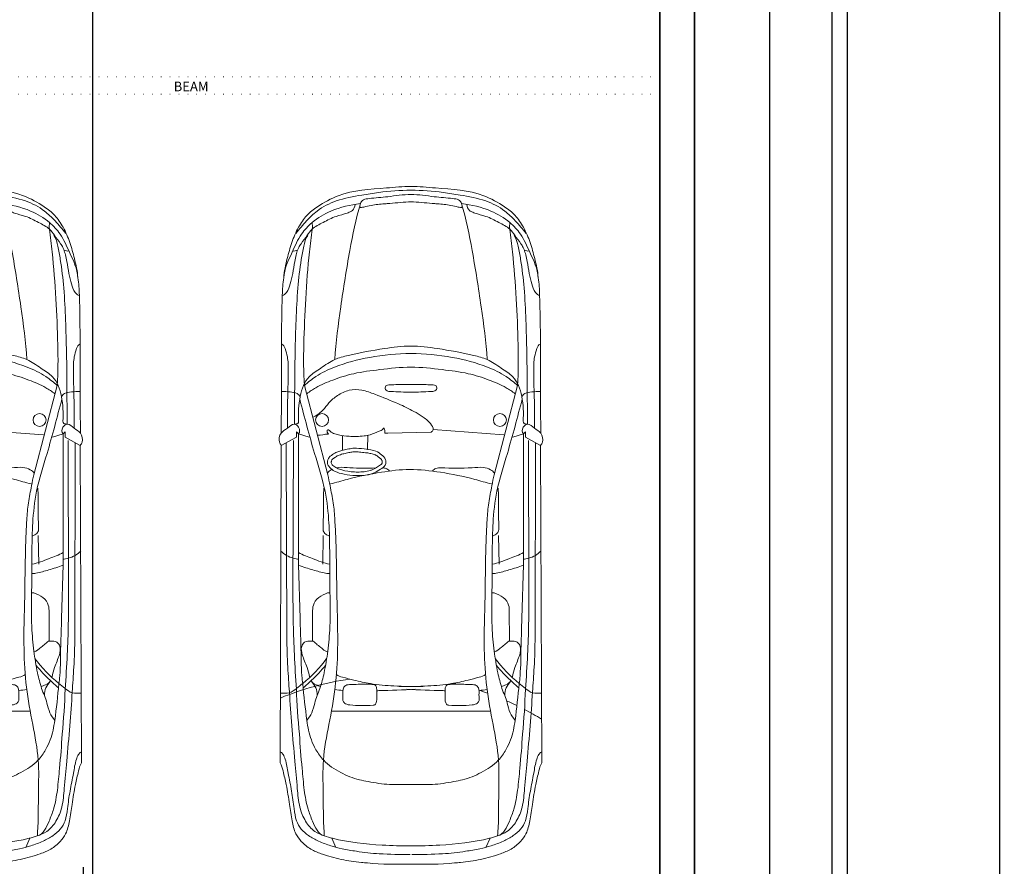
# Model space of a CAD drawing. Units: inches. Extents: x 1239 to 2276906, y 2273 to 321338.
# Tile 13 of 23: x 1754 to 2011, y 2429 to 2650. Entities that reach past the tile are written whole.
import ezdxf

# ---------------------------------------------------------------- set-up
doc = ezdxf.new("R2010")
doc.units = ezdxf.units.IN
doc.linetypes.add('DOT', pattern=[6.35, 0, -6.35])
for name, color, linetype, lineweight in [('A-ANNO-DIMS', 2, 'Continuous', 18), ('A-ANNO-TEXT', 7, 'Continuous', 18), ('BEAM LINE', 4, 'DOT', 18), ('C-PRKG', 8, 'Continuous', 13), ('C-PROP', 7, 'Continuous', 25), ('wall', 7, 'Continuous', 35)]:
    doc.layers.add(name, color=color, linetype=linetype, lineweight=lineweight)
doc.styles.get("Standard").update_dxf_attribs({"font": 'arial.ttf'})
doc.dimstyles.new('ISO-25', dxfattribs={"dimtxt": 4.5, "dimasz": 4, "dimexe": 1.25, "dimexo": 0.625, "dimtad": 1, "dimdec": 1, "dimlunit": 3, "dimtxsty": 'Standard', "dimcen": 2.5, "dimadec": 0, "dimazin": 0, "dimtfac": 1, "dimtdec": 1, "dimtmove": 0, "dimatfit": 3, "dimfxl": 1, "dimarcsym": 0})

# ---------------------------------------------------------------- blocks, each defined once
blk = doc.blocks.new('A$C242571DA')
for p, q in [((1659.9, 1632), (1714.3, 1732.5)), ((1699.9, 1699.4), (2984.7, 1695.8)), ((1714.3, 1732.5), (3817.1, 1739.9)), ((1638.3, 1618.5), (1625.1, 1632)), ((1625.1, 1632), (1659.9, 1632)), ((1681.8, 1651.6), (2695.2, 1655.3)), ((1317.4, 1579.7), (1909.8, 1424.9)), ((1638.3, 1618.5), (2503.3, 1618.5)), ((1659.9, 1548.1), (1638.3, 1618.5)), ((2503.3, 1618.5), (2861.6, 1607.5)), ((3007.2, 1526.5), (2808.1, 1525.2)), ((1644, 1489.1), (1610.4, 1020.2)), ((2311.9, 1454.3), (2500.6, 1456.9)), ((3474.6, 1401.1), (3474.6, 843)), ((4315.2, 1398), (4377.3, 1370.5)), ((1626.1, 1006.5), (1632.8, 719.7)), ((3474.6, 345.6), (3474.6, 903.8)), ((1740.2, 584.9), (1649.3, 586.9)), ((1746.1, 420.6), (1649.3, 420.6)), ((4315.2, 348.7), (4377.3, 376.3)), ((1317.4, 167), (1909.8, 321.9)), ((2311.9, 292.5), (2500.6, 289.8)), ((1659.9, 198.7), (1638.3, 128.2)), ((3007.2, 220.3), (2808.1, 221.6)), ((2503.3, 128.2), (2861.6, 139.2)), ((1638.3, 128.2), (1625.1, 114.7)), ((1625.1, 114.7), (1659.9, 114.7)), ((1638.3, 128.2), (2503.3, 128.2)), ((1659.9, 114.7), (1714.3, 14.2)), ((1681.8, 95.1), (2695.2, 91.4)), ((1699.9, 47.3), (2984.7, 51)), ((1714.3, 14.2), (3817.1, 6.9))]:
    blk.add_line(p, q)
for centre in [(1546.4, 1462.5), (1546.4, 284.2)]:
    blk.add_ellipse(centre, major_axis=(0, 42.9), ratio=0.983266, start_param=4.712389, end_param=10.995574)
for points, knots in [([(0, 873.4), (0, 927.8), (15.6, 1088.6), (25.5, 1309.8), (120.7, 1476.4), (189.2, 1569), (273.5, 1623.1), (369.9, 1666.3), (483, 1694.7), (561.3, 1714.9), (604.6, 1715.7)], [0, 0, 0, 0, 0.16039, 0.479033, 0.632967, 0.722015, 0.817474, 0.927562, 1.03733, 1.167094, 1.167094, 1.167094, 1.167094]), ([(604.6, 1715.7), (545.5, 1714.5), (448.5, 1664.6), (320.8, 1610.6), (225.4, 1521.2), (147.3, 1390.5), (121.7, 1275.2), (113.6, 1208.7)], [0, 0, 0, 0, 0.1772572, 0.3124951, 0.4151678, 0.5597243, 0.7575412, 0.7575412, 0.7575412, 0.7575412]), ([(722.7, 1726.6), (720.8, 1714.9), (694.5, 1689.9), (643, 1671.8), (573.6, 1655.4), (508.5, 1647), (455.2, 1634.7), (428.7, 1627.3), (416.9, 1624.1)], [0, 0, 0, 0, 0.034703, 0.0959761, 0.1659336, 0.2471559, 0.2929944, 0.3295918, 0.3295918, 0.3295918, 0.3295918]), ([(604.6, 1715.7), (642.1, 1723.4), (788.5, 1729.2), (1039.3, 1732.2), (1344.5, 1729.9), (1542, 1733.1), (1633.8, 1733.7)], [0, 0, 0, 0, 0.114897, 0.437061, 0.754269, 1.029686, 1.029686, 1.029686, 1.029686]), ([(1043.6, 1729.2), (1048.6, 1717.9), (1080.9, 1704.2), (1138.6, 1687.6), (1237.7, 1685.6), (1394.7, 1691.3), (1521.7, 1692.4), (1601.5, 1692.7)], [0, 0, 0, 0, 0.0364992, 0.0923739, 0.1867837, 0.3273982, 0.5667068, 0.5667068, 0.5667068, 0.5667068]), ([(1356.8, 1732.2), (1357.1, 1712.8), (1360, 1678.8), (1363.9, 1630.5), (1383.3, 1613.5), (1391, 1607.2)], [0, 0, 0, 0, 1.462159, 2.651105, 3.386321, 3.386321, 3.386321, 3.386321]), ([(1714.3, 1732.5), (1707.7, 1737.6), (1683.3, 1753), (1628.7, 1741.2), (1605.6, 1691.5), (1561.7, 1652.4), (1594.1, 1610.3), (1627.9, 1608.3), (1638.3, 1618.5)], [0, 0, 0, 0, 0.024864, 0.0846267, 0.1362471, 0.1900683, 0.2245199, 0.2681841, 0.2681841, 0.2681841, 0.2681841]), ([(2414.7, 1735), (2424.9, 1723.3), (2447.2, 1698.8), (2461.2, 1657.6), (2468.1, 1629), (2468, 1616.1)], [1.808086, 1.808086, 1.808086, 1.808086, 2.918874, 4.131288, 5.10151, 5.10151, 5.10151, 5.10151]), ([(3356.5, 1739.4), (3354.9, 1719.2), (3360.8, 1678.2), (3324, 1631.5), (3255.4, 1544.3), (3187.1, 1476.2), (3125.2, 1432.2)], [0, 0, 0, 0, 0.0597371, 0.1139981, 0.1672498, 0.3938869, 0.3938869, 0.3938869, 0.3938869]), ([(3745.3, 1736.8), (3748.5, 1730.1), (3764.2, 1717.1), (3811.5, 1698.6), (3894.7, 1686.7), (4002.9, 1663.2), (4107.9, 1648.7), (4195.8, 1638.3), (4258.6, 1603.2), (4302.1, 1549.7), (4339.9, 1483.8), (4365.2, 1407.6), (4389.6, 1324.4), (4397.9, 1266.9), (4401.8, 1235.2)], [0, 0, 0, 0, 0.0219205, 0.0572122, 0.1522539, 0.2718866, 0.3894011, 0.4710097, 0.5346344, 0.5986698, 0.6733118, 0.758696, 0.8351341, 0.9293726, 0.9293726, 0.9293726, 0.9293726]), ([(3817.1, 1739.9), (3833.2, 1729.7), (3882.9, 1718.2), (3973.3, 1695.2), (4085.1, 1680.5), (4193.8, 1662.8), (4280.6, 1644.3), (4343.9, 1598.1), (4390, 1540.3), (4427.4, 1448.7), (4457.8, 1336.6), (4475.7, 1233.4), (4478.4, 1175.1), (4479.3, 1161.6)], [0, 0, 0, 0, 0.056668, 0.14946, 0.28161, 0.392935, 0.481686, 0.542967, 0.622845, 0.69797, 0.833643, 0.965665, 1.00577, 1.00577, 1.00577, 1.00577]), ([(310.7, 1637.3), (282.5, 1613.7), (230.1, 1569.9), (148.7, 1486.2), (84.8, 1361.3), (60, 1219), (32.6, 1054.3), (25.1, 944.9), (25.1, 873.4)], [0, 0, 0, 0, 0.1095129, 0.2035347, 0.3452507, 0.5161382, 0.6275464, 0.8383798, 0.8383798, 0.8383798, 0.8383798]), ([(426.8, 1656.7), (428.5, 1646.6), (426.9, 1625), (399.8, 1616.6), (368.1, 1593.9), (328, 1564.6), (271.6, 1523.9), (237, 1451.9), (196.2, 1376.7), (183.8, 1314.9), (170, 1279.6), (157.2, 1254.2), (133.3, 1244.4), (118.6, 1242.9)], [0, 0, 0, 0, 0.0304541, 0.0502818, 0.0786089, 0.1479133, 0.1986294, 0.2831705, 0.3780326, 0.4523267, 0.4667809, 0.4902599, 0.5347198, 0.5347198, 0.5347198, 0.5347198]), ([(323.7, 1557.5), (344.8, 1571.9), (400.4, 1585.1), (516, 1606.8), (680.3, 1625.8), (885.4, 1635.7), (1116.8, 1642.2), (1346.1, 1644.2), (1504.7, 1644.7), (1574, 1645.7)], [0, 0, 0, 0, 0.076148, 0.165903, 0.355672, 0.569871, 0.782325, 1.050047, 1.257936, 1.257936, 1.257936, 1.257936]), ([(1574, 1645.7), (1572.9, 1638), (1574.1, 1622), (1559.9, 1618.7), (1555.2, 1617.8)], [0, 0, 0, 0, 0.02274132, 0.03717479, 0.03717479, 0.03717479, 0.03717479]), ([(2695.2, 1655.3), (2829.9, 1655.3), (3041.2, 1651.4), (3351.3, 1630.7), (3527.5, 1623.2), (3626.6, 1612)], [0, 0, 0, 0, 0.4042759, 0.6333827, 0.9326252, 0.9326252, 0.9326252, 0.9326252]), ([(2984.7, 1695.8), (3051, 1695.6), (3172.1, 1691.3), (3367.4, 1677.6), (3575.2, 1664.3), (3788.2, 1643.6), (3968, 1628.1), (4103.8, 1616.8), (4203.6, 1578.1), (4271.8, 1519.5), (4300.6, 1452.1), (4341.7, 1305.3), (4361.8, 1111.2), (4367.5, 936.8), (4367.5, 873.4)], [0, 0, 0, 0, 0.198873, 0.363323, 0.587433, 0.823543, 1.004622, 1.129816, 1.230113, 1.320655, 1.388577, 1.443334, 1.771447, 1.958652, 1.958652, 1.958652, 1.958652]), ([(1317.4, 1579.7), (1227.8, 1586.1), (1036, 1584.8), (741.2, 1572.5), (486.1, 1553.3), (333.3, 1534.3), (283.3, 1528.5)], [0, 0, 0, 0, 0.269375, 0.574535, 0.885339, 1.036319, 1.036319, 1.036319, 1.036319]), ([(1555.2, 1617.8), (1527.7, 1617.8), (1472.5, 1620.4), (1392.7, 1608.8), (1318.5, 1591), (1249.4, 1545.5), (1201.4, 1466.7), (1142.8, 1385.7), (1104.8, 1240.4), (1076, 1072.3), (1056.4, 932.4), (1056.4, 873.4)], [0, 0, 0, 0, 0.082256, 0.165174, 0.241383, 0.30939, 0.405348, 0.511507, 0.603349, 0.843635, 1.017671, 1.017671, 1.017671, 1.017671]), ([(1317.4, 1579.7), (1296.6, 1555.5), (1247.9, 1494.4), (1177.6, 1350.5), (1124.2, 1137.4), (1105.5, 964.9), (1105.5, 873.4)], [0, 0, 0, 0, 0.0947759, 0.2311242, 0.4700259, 0.7400315, 0.7400315, 0.7400315, 0.7400315]), ([(3535.9, 1563.1), (3520.1, 1550.9), (3484.4, 1526.1), (3408.2, 1510.9), (3323.4, 1473.1), (3207.9, 1445), (3072.6, 1422.2), (2866.9, 1404.6), (2626.4, 1412.9), (2396.7, 1410.8), (2200.9, 1416.9), (2001.3, 1438.2), (1732.1, 1525.9), (1527.9, 1578.9), (1407.5, 1610.7)], [0, 0, 0, 0, 0.05975, 0.126928, 0.230034, 0.336675, 0.482225, 0.641324, 0.954906, 1.203173, 1.330375, 1.542773, 1.802261, 2.175545, 2.175545, 2.175545, 2.175545]), ([(2424, 1618.7), (2441.5, 1589.9), (2464.2, 1518.9), (2495.4, 1450.9), (2501.6, 1411.3)], [0, 0, 0, 0, 0.1000351, 0.2184418, 0.2184418, 0.2184418, 0.2184418]), ([(2507.7, 1618.4), (2521, 1587.7), (2536.6, 1527.1), (2559.6, 1458.5), (2563.3, 1420.6), (2563.8, 1411.4)], [0, 0, 0, 0, 2.528586, 4.711885, 5.408215, 5.408215, 5.408215, 5.408215]), ([(2861.6, 1607.5), (2921.1, 1607.3), (3047.2, 1600.8), (3191.4, 1602), (3356.6, 1584.1), (3498.3, 1570.6), (3623.2, 1549.4), (3664.1, 1533.3)], [0, 0, 0, 0, 0.1783018, 0.3787173, 0.431954, 0.6762374, 0.8077184, 0.8077184, 0.8077184, 0.8077184]), ([(3248.1, 1545.2), (3226.9, 1550.4), (3176.1, 1562.1), (3113.7, 1592.9), (3052.6, 1605.3), (3010.4, 1578.8), (3010.3, 1545.3), (3010.3, 1515.9), (3033.7, 1500.1), (3052.6, 1465.2), (3078.9, 1443.5), (3084, 1424.4)], [0, 0, 0, 0, 0.0655106, 0.1550445, 0.2094604, 0.2438604, 0.287164, 0.3001388, 0.3275984, 0.3616951, 0.4200969, 0.4200969, 0.4200969, 0.4200969]), ([(3319, 1587.1), (3303.3, 1568.1), (3256.9, 1516.7), (3206.7, 1467.3), (3171.4, 1439.5)], [0, 0, 0, 0, 1.868162, 5.271297, 5.271297, 5.271297, 5.271297]), ([(3626.6, 1612), (3702.5, 1609.1), (3826.2, 1596.8), (3991.4, 1583.2), (4111.7, 1562.4), (4212.2, 1522.7), (4290.4, 1488), (4300.7, 1447.5)], [0, 0, 0, 0, 0.2277977, 0.3719478, 0.4996814, 0.5863441, 0.709615, 0.709615, 0.709615, 0.709615]), ([(1372.8, 1563.1), (1357.2, 1545), (1321.6, 1490.1), (1277, 1385.7), (1232.8, 1244.2), (1211.1, 1069.4), (1196.8, 942.4), (1196.8, 873.4)], [0, 0, 0, 0, 0.0708922, 0.1925846, 0.3348457, 0.5072814, 0.7109928, 0.7109928, 0.7109928, 0.7109928]), ([(2808.1, 1525.2), (2791.9, 1525.1), (2751.9, 1519.7), (2710.6, 1472.6), (2690, 1431.1), (2690.5, 1409.6)], [0, 0, 0, 0, 0.0486628, 0.1144515, 0.1777721, 0.1777721, 0.1777721, 0.1777721]), ([(3275.5, 1532.8), (3287.5, 1528.3), (3299.8, 1504.9), (3308.4, 1482.5), (3311.7, 1472.6)], [0, 0, 0, 0, 0.983949, 1.771691, 1.771691, 1.771691, 1.771691]), ([(3372.2, 1495.3), (3354.4, 1496.8), (3316, 1494.7), (3291.6, 1525.8), (3275.5, 1532.8)], [0, 0, 0, 0, 0.0535488, 0.1060573, 0.1060573, 0.1060573, 0.1060573]), ([(3664.1, 1533.3), (3687, 1526), (3734.8, 1502.3), (3816.7, 1444.8), (3884.1, 1342.9), (3925.1, 1239.9), (3937.3, 1177), (3940.4, 1157.6)], [0, 0, 0, 0, 0.0720749, 0.1581284, 0.2958089, 0.4262456, 0.4842292, 0.4842292, 0.4842292, 0.4842292]), ([(1909.8, 1424.9), (1933.5, 1418.7), (1995.6, 1407.6), (2094.4, 1385.8), (2211.8, 1377.1), (2419, 1366.9), (2704.7, 1366.5), (3032.7, 1354.2), (3316.2, 1371), (3558.7, 1415.9), (3789.1, 1461.7), (4028.9, 1452.9), (4196.2, 1455.2), (4292.7, 1447.9), (4300.7, 1447.5)], [0, 0, 0, 0, 0.073325, 0.188896, 0.303039, 0.425821, 0.811242, 1.159737, 1.41058, 1.660623, 1.899627, 2.11145, 2.377727, 2.401703, 2.401703, 2.401703, 2.401703]), ([(1997.2, 1450.5), (2039.7, 1454.5), (2126.7, 1451.9), (2219.8, 1454.5), (2287.1, 1456.9), (2305.7, 1434.4), (2313.2, 1419.9), (2315.8, 1413.5)], [0, 0, 0, 0, 3.267856, 6.568708, 7.399663, 8.099385, 8.621705, 8.621705, 8.621705, 8.621705]), ([(113.6, 1208.7), (215.2, 1238.6), (443.2, 1284.9), (788, 1338.7), (1029.5, 1370.7), (1146.4, 1378.6)], [0, 0, 0, 0, 0.317374, 0.69576, 1.04714, 1.04714, 1.04714, 1.04714]), ([(1898.5, 1426.2), (1889, 1420.6), (1871, 1397.2), (1856.4, 1345.2), (1867.7, 1233.5), (1864.3, 1132.3), (1863, 1038.5), (1876.9, 1022.3), (1884.5, 1015.7)], [0, 0, 0, 0, 0.842998, 2.122875, 3.997599, 9.174838, 10.012722, 10.751336, 10.751336, 10.751336, 10.751336]), ([(1969.6, 1407.3), (1960.5, 1369.8), (1927, 1259.1), (1890.9, 1078.4), (1874.3, 933), (1874.3, 864.4)], [0, 0, 0, 0, 0.1139079, 0.3411539, 0.543502, 0.543502, 0.543502, 0.543502]), ([(3231.5, 1368.3), (3240.8, 1356.2), (3253.1, 1315.7), (3271.9, 1240.7), (3297.9, 1127.9), (3310.5, 974.6), (3311.2, 858.3), (3311.6, 794.4)], [0, 0, 0, 0, 0.0451009, 0.1211996, 0.2308505, 0.385263, 0.5739042, 0.5739042, 0.5739042, 0.5739042]), ([(3294.8, 1174.5), (3294.8, 1207.4), (3299.6, 1249.5), (3298.3, 1303.9), (3326.3, 1329), (3363.9, 1320.7), (3399.3, 1329.3), (3422.1, 1315.7), (3430.7, 1297.9), (3438.7, 1234.2), (3439.6, 1174.4), (3434.7, 1112.2), (3418.9, 1102), (3395.9, 1098.6), (3362.6, 1100.9), (3331.1, 1096.6), (3298.8, 1107.6), (3297.3, 1140.3), (3294.8, 1160.9), (3294.8, 1174.5)], [0, 0, 0, 0, 0.0969044, 0.1295913, 0.1506192, 0.1985921, 0.2360698, 0.2557908, 0.2719711, 0.2929882, 0.44406, 0.4519132, 0.4720918, 0.4918599, 0.5228758, 0.5707096, 0.5892096, 0.6145759, 0.654681, 0.654681, 0.654681, 0.654681]), ([(113.6, 1208.7), (103.3, 1207), (83.6, 1187.6), (76.5, 1122.2), (68.2, 1017.3), (53.4, 925), (53.4, 873.4)], [0, 0, 0, 0, 0.0314754, 0.0702057, 0.1915753, 0.3439346, 0.3439346, 0.3439346, 0.3439346]), ([(135.5, 1213.1), (139.1, 1211.8), (138.4, 1193.3), (132.6, 1168.3), (118.8, 1111.9), (115.6, 1058.9), (109, 974.6), (102.4, 920.1), (102.4, 873.4)], [0, 0, 0, 0, 0.0114788, 0.0403472, 0.0875838, 0.1755608, 0.1991501, 0.3369659, 0.3369659, 0.3369659, 0.3369659]), ([(4401.8, 1235.2), (4411.9, 1185.3), (4421.6, 1065.8), (4424.1, 946.5), (4424.1, 878)], [0, 0, 0, 0, 0.1502861, 0.3522699, 0.3522699, 0.3522699, 0.3522699]), ([(3940.4, 1157.6), (3949.9, 1111), (3964.3, 1016.4), (3960.5, 921), (3959.8, 873.4)], [0, 0, 0, 0, 0.140379, 0.2808468, 0.2808468, 0.2808468, 0.2808468]), ([(1311.3, 873.4), (1311.2, 902.4), (1309.2, 950.9), (1315, 1002.2), (1314.2, 1039.4), (1332.1, 1044.9), (1345.7, 1044.2), (1356.8, 1028.5), (1359.2, 970.2), (1361.5, 917.6), (1362.9, 873.4)], [0, 0, 0, 0, 0.0857277, 0.1381048, 0.1641986, 0.1769751, 0.1890325, 0.2028129, 0.2286049, 0.3592554, 0.3592554, 0.3592554, 0.3592554]), ([(3339.2, 1099), (3339.1, 1094.8), (3336.4, 1010.6), (3333.2, 926.3), (3330, 846.2)], [11.235438, 11.235438, 11.235438, 11.235438, 11.552536, 17.586883, 17.586883, 17.586883, 17.586883]), ([(1626.1, 1006.5), (1623.5, 1013), (1603.1, 1029.4), (1559.1, 995), (1523, 951.9), (1480.3, 878.3), (1430.5, 774.3), (1385.5, 658.5), (1343.7, 551.3), (1343, 461.7), (1380.3, 386.9), (1428.2, 329.9), (1480.1, 294.6), (1509.8, 257.4), (1524.8, 232.6), (1528, 222.1)], [0, 0, 0, 0, 0.527288, 1.647451, 3.487558, 5.099073, 7.968657, 12.238313, 14.475187, 16.613757, 18.744202, 20.639343, 22.223389, 23.452731, 24.286529, 24.286529, 24.286529, 24.286529]), ([(3231.5, 378.5), (3240.8, 390.5), (3253.1, 431), (3271.9, 506.1), (3297.9, 618.9), (3310.5, 772.1), (3311.2, 888.4), (3311.6, 952.4)], [0, 0, 0, 0, 0.0451009, 0.1211996, 0.2308505, 0.385263, 0.5739042, 0.5739042, 0.5739042, 0.5739042]), ([(0, 873.4), (0, 819), (15.6, 658.1), (25.5, 437), (120.7, 270.3), (189.2, 177.8), (273.5, 123.7), (369.9, 80.4), (483, 52), (561.3, 31.9), (604.6, 31)], [0, 0, 0, 0, 0.16039, 0.479033, 0.632967, 0.722015, 0.817474, 0.927562, 1.03733, 1.167094, 1.167094, 1.167094, 1.167094]), ([(310.7, 109.5), (282.5, 133.1), (230.1, 176.9), (148.7, 260.5), (84.8, 385.5), (60, 527.8), (32.6, 692.4), (25.1, 801.9), (25.1, 873.4)], [0, 0, 0, 0, 0.1095129, 0.2035347, 0.3452507, 0.5161382, 0.6275464, 0.8383798, 0.8383798, 0.8383798, 0.8383798]), ([(113.6, 538.1), (103.3, 539.8), (83.6, 559.2), (76.5, 624.5), (68.2, 729.4), (53.4, 821.7), (53.4, 873.4)], [0, 0, 0, 0, 0.0314754, 0.0702057, 0.1915753, 0.3439346, 0.3439346, 0.3439346, 0.3439346]), ([(135.5, 533.6), (139.1, 534.9), (138.4, 553.4), (132.6, 578.4), (118.8, 634.9), (115.6, 687.8), (109, 772.2), (102.4, 826.7), (102.4, 873.4)], [0, 0, 0, 0, 0.0114788, 0.0403472, 0.0875838, 0.1755608, 0.1991501, 0.3369659, 0.3369659, 0.3369659, 0.3369659]), ([(1555.2, 129), (1527.7, 129), (1472.5, 126.3), (1392.7, 138), (1318.5, 155.7), (1249.4, 201.3), (1201.4, 280.1), (1142.8, 361.1), (1104.8, 506.4), (1076, 674.5), (1056.4, 814.4), (1056.4, 873.4)], [0, 0, 0, 0, 0.082256, 0.165174, 0.241383, 0.30939, 0.405348, 0.511507, 0.603349, 0.843635, 1.017671, 1.017671, 1.017671, 1.017671]), ([(1317.4, 167), (1296.6, 191.2), (1247.9, 252.4), (1177.6, 396.3), (1124.2, 609.4), (1105.5, 781.8), (1105.5, 873.4)], [0, 0, 0, 0, 0.0947759, 0.2311242, 0.4700259, 0.7400315, 0.7400315, 0.7400315, 0.7400315]), ([(1372.8, 183.6), (1357.2, 201.8), (1321.6, 256.7), (1277, 361), (1232.8, 502.6), (1211.1, 677.3), (1196.8, 804.3), (1196.8, 873.4)], [0, 0, 0, 0, 0.0708922, 0.1925846, 0.3348457, 0.5072814, 0.7109928, 0.7109928, 0.7109928, 0.7109928]), ([(1311.3, 873.4), (1311.2, 844.3), (1309.2, 795.8), (1315, 744.6), (1314.2, 707.4), (1332.1, 701.9), (1345.7, 702.6), (1356.8, 718.2), (1359.2, 776.6), (1361.5, 829.1), (1362.9, 873.4)], [0, 0, 0, 0, 0.0857277, 0.1381048, 0.1641986, 0.1769751, 0.1890325, 0.2028129, 0.2286049, 0.3592554, 0.3592554, 0.3592554, 0.3592554]), ([(1969.6, 339.5), (1960.5, 377), (1926.9, 487.6), (1892.9, 662.7), (1874.3, 801.8), (1874.3, 864.4)], [0, 0, 0, 0, 0.1139079, 0.3411539, 0.5260188, 0.5260188, 0.5260188, 0.5260188]), ([(2984.7, 51), (3051, 51.1), (3172.1, 55.5), (3367.4, 69.2), (3575.2, 82.5), (3788.2, 103.1), (3968, 118.7), (4103.8, 130), (4203.6, 168.6), (4271.8, 227.3), (4300.6, 294.7), (4341.7, 441.5), (4361.8, 635.5), (4367.5, 809.9), (4367.5, 873.4)], [0, 0, 0, 0, 0.198873, 0.363323, 0.587433, 0.823543, 1.004622, 1.129816, 1.230113, 1.320655, 1.388577, 1.443334, 1.771447, 1.958652, 1.958652, 1.958652, 1.958652]), ([(3339.2, 647.8), (3339.1, 652), (3336.4, 736.2), (3333.2, 820.5), (3330, 900.6)], [11.235438, 11.235438, 11.235438, 11.235438, 11.552536, 17.586883, 17.586883, 17.586883, 17.586883]), ([(3940.4, 589.1), (3949.9, 635.7), (3964.3, 730.4), (3960.5, 825.8), (3959.8, 873.4)], [0, 0, 0, 0, 0.140379, 0.2808468, 0.2808468, 0.2808468, 0.2808468]), ([(4401.8, 511.5), (4411.9, 561.5), (4421.6, 681), (4424.1, 800.3), (4424.1, 868.8)], [0, 0, 0, 0, 0.1502861, 0.3522699, 0.3522699, 0.3522699, 0.3522699]), ([(1639.2, 326.1), (1635.3, 323.6), (1629, 318.4), (1613.1, 314.9), (1612, 324.2), (1613.2, 330.4), (1619, 337.5), (1629, 345.7), (1637.9, 366.1), (1649, 404.8), (1656.3, 472.9), (1656.2, 543.1), (1644.6, 610.9), (1623, 651.2), (1615, 684.3), (1598.5, 691.2), (1604, 696.6), (1610.3, 699.7), (1618.8, 698.9), (1625.9, 701.3), (1638.1, 698.6), (1633, 713.4), (1632.8, 719.7)], [0, 0, 0, 0, 0.0138597, 0.0278304, 0.0329137, 0.0379971, 0.0465756, 0.0592704, 0.0762214, 0.1105991, 0.1789801, 0.2766959, 0.3173629, 0.3800771, 0.4110544, 0.4160421, 0.4210284, 0.4277212, 0.4387433, 0.4448131, 0.4508005, 0.4694463, 0.4694463, 0.4694463, 0.4694463]), ([(1863.4, 685.6), (1863.6, 693.5), (1865.3, 711), (1876.9, 724.5), (1884.5, 731)], [9.436432, 9.436432, 9.436432, 9.436432, 10.012722, 10.751336, 10.751336, 10.751336, 10.751336]), ([(1740.2, 584.9), (1737.8, 571.7), (1749.5, 644.3), (1766.4, 664.5), (1792.2, 700.2), (1821.5, 709.7), (1853.1, 703.9), (1874, 668.4), (1904.5, 622.6), (1915.6, 557.2), (1915.1, 484.2), (1905.7, 417.6), (1884.9, 362.8), (1859.3, 329.1), (1831.3, 318.1), (1810.8, 322.7), (1792.2, 329.3), (1777.9, 350.3), (1753, 385.9), (1737.9, 465.8), (1728.8, 497.3), (1742.4, 597.6), (1740.2, 584.9)], [0, 0, 0, 0, 0.03969, 0.089634, 0.13125, 0.1542862, 0.1797268, 0.2207266, 0.2680991, 0.3447665, 0.4095645, 0.4843001, 0.541515, 0.5817687, 0.6060665, 0.6262474, 0.6436722, 0.6634686, 0.6988791, 0.7758465, 0.8696394, 0.907731, 0.907731, 0.907731, 0.907731]), ([(1764.9, 587), (1765.6, 590.8), (1766.4, 595.5), (1768.5, 605.7), (1769.7, 611.3), (1773.4, 626.6), (1775.6, 633), (1779.7, 642.1), (1781.6, 644.9), (1785.7, 650.6), (1787.1, 652.5), (1793, 660.3), (1797.4, 666.2), (1804.2, 673.7), (1806.8, 676.1), (1811.1, 679.4), (1812.9, 680.5), (1816.8, 682.1), (1818.8, 682.7), (1824.4, 683.5), (1828.3, 683.2), (1832.5, 682), (1833.6, 681.5), (1836, 680.2), (1837.9, 678.7), (1842.4, 673.7), (1844.9, 670.1), (1850.3, 661.7), (1853.4, 656.6), (1859.3, 647.3), (1862.1, 642.8), (1868.3, 632.6), (1871.4, 626.9), (1876.7, 615.7), (1878.9, 609.8), (1882.8, 597.4), (1884.4, 590.8), (1888.3, 570.5), (1889.7, 556.1), (1891.2, 527.4), (1891.1, 513.1), (1888.9, 470), (1885.1, 441.2), (1874.3, 404), (1870.6, 393.8), (1863.5, 378.7), (1860.6, 373.4), (1854.4, 363.6), (1851.2, 359.2), (1845, 352.6), (1842, 350.2), (1835.8, 346.4), (1832.6, 345.3), (1828.8, 344.6), (1827.9, 344.6), (1824.6, 344.9), (1822.6, 345.2), (1817.8, 346.4), (1814.9, 347.3), (1810.9, 348.7), (1809.4, 349.4), (1808.3, 350.1), (1808.1, 350.2), (1807.3, 351), (1806.7, 351.6), (1804.7, 354), (1803.1, 356.2), (1799.6, 361.3), (1798, 363.7), (1794.9, 368.2), (1793.4, 370.4), (1789.2, 376.9), (1786.7, 381), (1782.4, 389.3), (1780.5, 393.6), (1776.9, 403), (1775.2, 408), (1770.7, 423.5), (1768.3, 434.2), (1764.9, 450.5), (1763.6, 456.4), (1761.4, 466.8), (1760.4, 471.4), (1758.1, 484.4), (1757.3, 492.6), (1757.5, 510.7), (1757.8, 516.5), (1758.6, 528.4), (1759.1, 534.3), (1761.1, 553.9), (1763.1, 570.6), (1764.4, 581.5), (1764.6, 583), (1764.7, 585), (1764.8, 585.5), (1764.8, 586.5), (1764.8, 586.7), (1764.9, 587)], [0.497033, 0.497033, 0.497033, 0.497033, 0.723444, 0.723444, 0.974636, 0.974636, 1.50964, 1.50964, 2.044645, 2.044645, 2.271061, 2.271061, 2.862376, 2.862376, 3.217654, 3.217654, 3.537253, 3.537253, 3.856852, 3.856852, 4.368613, 4.368613, 4.584627, 4.584627, 4.99269, 4.99269, 5.400753, 5.400753, 5.808816, 5.808816, 6.216879, 6.216879, 6.778716, 6.778716, 7.350371, 7.350371, 7.922025, 7.922025, 9.065335, 9.065335, 10.208644, 10.208644, 12.495263, 12.495263, 13.409896, 13.409896, 13.929088, 13.929088, 14.44828, 14.44828, 14.909885, 14.909885, 15.371489, 15.371489, 15.62524, 15.62524, 15.87899, 15.87899, 16.120875, 16.120875, 16.36276, 16.36276, 16.51635, 16.51635, 16.669941, 16.669941, 16.921521, 16.921521, 17.136676, 17.136676, 17.351831, 17.351831, 17.782142, 17.782142, 18.204974, 18.204974, 18.627807, 18.627807, 19.473473, 19.473473, 19.978923, 19.978923, 20.484372, 20.484372, 21.475119, 21.475119, 21.859144, 21.859144, 22.162884, 22.162884, 22.770362, 22.770362, 22.900493, 22.900493, 22.951221, 22.951221, 22.964298, 22.964298, 22.964298, 22.964298]), ([(1863.7, 379.4), (1862.6, 384.2), (1857.6, 413.7), (1866.5, 501.6), (1865.2, 581.4), (1864.1, 639.5)], [1.749253, 1.749253, 1.749253, 1.749253, 2.122875, 3.997599, 8.307432, 8.307432, 8.307432, 8.307432]), ([(3294.8, 572.3), (3294.8, 539.4), (3299.6, 497.2), (3298.3, 442.9), (3326.3, 417.8), (3363.9, 426), (3399.3, 417.5), (3422.1, 431), (3430.7, 448.9), (3438.7, 512.5), (3439.6, 572.4), (3434.7, 634.6), (3418.9, 644.7), (3395.9, 648.2), (3362.6, 645.9), (3331.1, 650.1), (3298.8, 639.2), (3297.3, 606.5), (3294.8, 585.9), (3294.8, 572.3)], [0, 0, 0, 0, 0.0969044, 0.1295913, 0.1506192, 0.1985921, 0.2360698, 0.2557908, 0.2719711, 0.2929882, 0.44406, 0.4519132, 0.4720918, 0.4918599, 0.5228758, 0.5707096, 0.5892096, 0.6145759, 0.654681, 0.654681, 0.654681, 0.654681]), ([(3664.1, 213.5), (3687, 220.8), (3734.8, 244.4), (3816.7, 302), (3884.1, 403.8), (3925.1, 506.9), (3937.3, 569.7), (3940.4, 589.1)], [0, 0, 0, 0, 0.0720749, 0.1581284, 0.2958089, 0.4262456, 0.4842292, 0.4842292, 0.4842292, 0.4842292]), ([(604.6, 31), (545.5, 32.3), (448.5, 82.2), (320.8, 136.1), (225.4, 225.5), (147.3, 356.2), (121.7, 471.5), (113.6, 538.1)], [0, 0, 0, 0, 0.1772572, 0.3124951, 0.4151678, 0.5597243, 0.7575412, 0.7575412, 0.7575412, 0.7575412]), ([(113.6, 538.1), (215.2, 508.2), (443.2, 461.9), (788, 408.1), (1029.5, 376), (1146.4, 368.2)], [0, 0, 0, 0, 0.317374, 0.69576, 1.04714, 1.04714, 1.04714, 1.04714]), ([(3817.1, 6.9), (3833.2, 17), (3882.9, 28.6), (3973.3, 51.5), (4085.1, 66.3), (4193.8, 84), (4280.6, 102.4), (4343.9, 148.6), (4390, 206.4), (4427.4, 298), (4457.8, 410.1), (4475.7, 513.3), (4478.4, 571.6), (4479.3, 585.2)], [0, 0, 0, 0, 0.056668, 0.14946, 0.28161, 0.392935, 0.481686, 0.542967, 0.622845, 0.69797, 0.833643, 0.965665, 1.00577, 1.00577, 1.00577, 1.00577]), ([(426.8, 90), (428.5, 100.2), (426.9, 121.8), (399.8, 130.1), (368.1, 152.8), (328, 182.2), (271.6, 222.8), (237, 294.9), (196.2, 370.1), (183.8, 431.9), (170, 467.2), (157.2, 492.6), (133.3, 502.4), (118.6, 503.9)], [0, 0, 0, 0, 0.0304541, 0.0502818, 0.0786089, 0.1479133, 0.1986294, 0.2831705, 0.3780326, 0.4523267, 0.4667809, 0.4902599, 0.5347198, 0.5347198, 0.5347198, 0.5347198]), ([(3745.3, 10), (3748.5, 16.7), (3764.2, 29.7), (3811.5, 48.1), (3894.7, 60.1), (4002.9, 83.6), (4107.9, 98), (4195.8, 108.4), (4258.6, 143.5), (4302.1, 197), (4339.9, 262.9), (4365.2, 339.2), (4389.6, 422.4), (4397.9, 479.8), (4401.8, 511.5)], [0, 0, 0, 0, 0.0219205, 0.0572122, 0.1522539, 0.2718866, 0.3894011, 0.4710097, 0.5346344, 0.5986698, 0.6733118, 0.758696, 0.8351341, 0.9293726, 0.9293726, 0.9293726, 0.9293726]), ([(3535.9, 183.7), (3520.1, 195.9), (3484.4, 220.6), (3408.2, 235.8), (3323.4, 273.7), (3207.9, 301.8), (3072.6, 324.6), (2866.9, 342.1), (2626.4, 333.8), (2396.7, 335.9), (2200.9, 329.9), (2001.3, 308.6), (1732.1, 220.8), (1527.9, 167.8), (1407.5, 136)], [0, 0, 0, 0, 0.05975, 0.126928, 0.230034, 0.336675, 0.482225, 0.641324, 0.954906, 1.203173, 1.330375, 1.542773, 1.802261, 2.175545, 2.175545, 2.175545, 2.175545]), ([(1898.5, 320.6), (1889, 326.2), (1880.8, 336.8), (1874.8, 348.3), (1874, 349.7)], [0, 0, 0, 0, 0.8429982, 0.9626806, 0.9626806, 0.9626806, 0.9626806]), ([(1909.8, 321.9), (1933.5, 328.1), (1995.6, 339.2), (2094.4, 361), (2211.8, 369.6), (2419, 379.8), (2704.7, 380.3), (3032.7, 392.6), (3316.2, 375.8), (3558.7, 330.9), (3789.1, 285.1), (4028.9, 293.9), (4196.2, 291.5), (4292.7, 298.8), (4300.7, 299.2)], [0, 0, 0, 0, 0.073325, 0.188896, 0.303039, 0.425821, 0.811242, 1.159737, 1.41058, 1.660623, 1.899627, 2.11145, 2.377727, 2.401703, 2.401703, 2.401703, 2.401703]), ([(1997.2, 296.3), (2039.7, 292.2), (2126.7, 294.9), (2219.8, 292.3), (2287.1, 289.9), (2305.7, 312.3), (2313.2, 326.9), (2315.8, 333.2)], [0, 0, 0, 0, 3.267856, 6.568708, 7.399663, 8.099385, 8.621705, 8.621705, 8.621705, 8.621705]), ([(2424, 128), (2441.5, 156.9), (2464.2, 227.8), (2495.4, 295.8), (2501.6, 335.5)], [0, 0, 0, 0, 0.1000351, 0.2184418, 0.2184418, 0.2184418, 0.2184418]), ([(2507.7, 128.3), (2521, 159.1), (2536.6, 219.7), (2559.6, 288.3), (2563.3, 326.1), (2563.8, 335.3)], [0, 0, 0, 0, 2.528586, 4.711885, 5.408215, 5.408215, 5.408215, 5.408215]), ([(2808.1, 221.6), (2791.9, 221.6), (2751.9, 227.1), (2710.6, 274.2), (2690, 315.7), (2690.5, 337.1)], [0, 0, 0, 0, 0.0486628, 0.1144515, 0.1777721, 0.1777721, 0.1777721, 0.1777721]), ([(3248.1, 201.6), (3226.9, 196.3), (3176.1, 184.7), (3113.7, 153.8), (3052.6, 141.4), (3010.4, 168), (3010.3, 201.5), (3010.3, 230.9), (3033.7, 246.6), (3052.6, 281.6), (3078.9, 303.2), (3084, 322.4)], [0, 0, 0, 0, 0.0655106, 0.1550445, 0.2094604, 0.2438604, 0.287164, 0.3001388, 0.3275984, 0.3616951, 0.4200969, 0.4200969, 0.4200969, 0.4200969]), ([(3356.5, 7.4), (3354.9, 27.5), (3360.8, 68.5), (3324, 115.2), (3255.4, 202.5), (3187.1, 270.5), (3125.2, 314.6)], [0, 0, 0, 0, 0.0597371, 0.1139981, 0.1672498, 0.3938869, 0.3938869, 0.3938869, 0.3938869]), ([(3319, 159.7), (3303.3, 178.6), (3256.9, 230), (3206.7, 279.5), (3171.4, 307.2)], [0, 0, 0, 0, 1.868162, 5.271297, 5.271297, 5.271297, 5.271297]), ([(3275.5, 214), (3287.5, 218.5), (3299.8, 241.9), (3308.4, 264.3), (3311.7, 274.2)], [0, 0, 0, 0, 0.983949, 1.771691, 1.771691, 1.771691, 1.771691]), ([(3626.6, 134.7), (3702.5, 137.7), (3826.2, 149.9), (3991.4, 163.5), (4111.7, 184.4), (4212.2, 224.1), (4290.4, 258.8), (4300.7, 299.2)], [0, 0, 0, 0, 0.2277977, 0.3719478, 0.4996814, 0.5863441, 0.709615, 0.709615, 0.709615, 0.709615]), ([(1317.4, 167), (1227.8, 160.7), (1036, 161.9), (741.2, 174.2), (486.1, 193.4), (333.3, 212.5), (283.3, 218.3)], [0, 0, 0, 0, 0.269375, 0.574535, 0.885339, 1.036319, 1.036319, 1.036319, 1.036319]), ([(2861.6, 139.2), (2921.1, 139.4), (3047.2, 146), (3191.4, 144.8), (3356.6, 162.6), (3498.3, 176.1), (3623.2, 197.4), (3664.1, 213.5)], [0, 0, 0, 0, 0.1783018, 0.3787173, 0.431954, 0.6762374, 0.8077184, 0.8077184, 0.8077184, 0.8077184]), ([(3372.2, 251.5), (3354.4, 249.9), (3316, 252), (3291.6, 220.9), (3275.5, 214)], [0, 0, 0, 0, 0.0535488, 0.1060573, 0.1060573, 0.1060573, 0.1060573]), ([(323.7, 189.2), (344.8, 174.9), (400.4, 161.7), (516, 139.9), (680.3, 121), (885.4, 111), (1116.8, 104.5), (1346.1, 102.5), (1504.7, 102), (1574, 101.1)], [0, 0, 0, 0, 0.076148, 0.165903, 0.355672, 0.569871, 0.782325, 1.050047, 1.257936, 1.257936, 1.257936, 1.257936]), ([(1356.8, 14.5), (1357.1, 33.9), (1360, 68), (1363.9, 116.3), (1383.3, 133.2), (1391, 139.5)], [0, 0, 0, 0, 1.462159, 2.651105, 3.386321, 3.386321, 3.386321, 3.386321]), ([(1714.3, 14.2), (1707.7, 9.2), (1683.3, -6.3), (1628.7, 5.5), (1605.6, 55.3), (1561.7, 94.4), (1594.1, 136.5), (1627.9, 138.5), (1638.3, 128.2)], [0, 0, 0, 0, 0.024864, 0.0846267, 0.1362471, 0.1900683, 0.2245199, 0.2681841, 0.2681841, 0.2681841, 0.2681841]), ([(2414.7, 11.8), (2424.9, 23.5), (2447.2, 48), (2461.2, 89.1), (2468.1, 117.8), (2468, 130.7)], [1.808086, 1.808086, 1.808086, 1.808086, 2.918874, 4.131288, 5.10151, 5.10151, 5.10151, 5.10151]), ([(2695.2, 91.4), (2829.9, 91.5), (3041.2, 95.4), (3351.3, 116.1), (3527.5, 123.5), (3626.6, 134.7)], [0, 0, 0, 0, 0.4042759, 0.6333827, 0.9326252, 0.9326252, 0.9326252, 0.9326252]), ([(722.7, 20.2), (720.8, 31.8), (694.5, 56.8), (643, 75), (573.6, 91.4), (508.5, 99.8), (455.2, 112.1), (428.7, 119.5), (416.9, 122.6)], [0, 0, 0, 0, 0.034703, 0.0959761, 0.1659336, 0.2471559, 0.2929944, 0.3295918, 0.3295918, 0.3295918, 0.3295918]), ([(1574, 101.1), (1572.9, 108.7), (1574.1, 124.8), (1559.9, 128), (1555.2, 129)], [0, 0, 0, 0, 0.02274132, 0.03717479, 0.03717479, 0.03717479, 0.03717479]), ([(604.6, 31), (642.1, 23.4), (788.5, 17.5), (1039.3, 14.6), (1344.5, 16.8), (1542, 13.6), (1633.8, 13.1)], [0, 0, 0, 0, 0.114897, 0.437061, 0.754269, 1.029686, 1.029686, 1.029686, 1.029686]), ([(1043.6, 17.6), (1048.6, 28.9), (1080.9, 42.6), (1138.6, 59.2), (1237.7, 61.2), (1394.7, 55.4), (1521.7, 54.3), (1601.5, 54.1)], [0, 0, 0, 0, 0.0364992, 0.0923739, 0.1867837, 0.3273982, 0.5667068, 0.5667068, 0.5667068, 0.5667068])]:
    blk.add_open_spline(points, degree=3, knots=knots)
for points in [[(283.3, 1528.5), (267.8, 1524.6), (251.4, 1527.5), (235.4, 1528.5)], [(3331.9, 1378.1), (3334.2, 1360.4), (3335.9, 1342.5), (3337.3, 1324.5)], [(4479.3, 1161.6), (4491, 1066.2), (4488, 969.5), (4488, 873.4)], [(4479.3, 585.2), (4491, 680.6), (4488, 777.3), (4488, 873.4)], [(3331.9, 368.6), (3334.2, 386.4), (3335.9, 404.3), (3337.3, 422.2)], [(1646.2, 253.1), (1647.8, 277.5), (1640, 301.6), (1639.2, 326.1)], [(283.3, 218.3), (267.8, 222.1), (251.4, 219.2), (235.4, 218.3)]]:
    blk.add_open_spline(points, degree=3)
blk = doc.blocks.new('*D38')
at = {"layer": 'A-ANNO-DIMS', "color": 0, "lineweight": -2, "transparency": 16777216}
for p, q in [((1971.01, 3545.9), (2011.25, 3545.9)), ((2010, 3541.9), (2010, 2342.75)), ((1971.01, 2338.75), (2011.25, 2338.75))]:
    blk.add_line(p, q, dxfattribs=at)
at = {"layer": 'A-ANNO-DIMS', "color": 0, "transparency": 16777216}
for points in [[(2009.33, 3541.9), (2010.67, 3541.9), (2010, 3545.9)], [(2009.33, 2342.75), (2010.67, 2342.75), (2010, 2338.75)]]:
    blk.add_solid(points, dxfattribs=at)
at = {"layer": 'Defpoints', "color": 0, "transparency": 16777216}
for p in [(1970.38, 3545.9), (1970.38, 2338.75), (2010, 2338.75)]:
    blk.add_point(p, dxfattribs=at)
at = {"layer": 'A-ANNO-DIMS', "color": 0, "transparency": 16777216, "insert": (2007.08, 2942.32), "char_height": 4.5, "attachment_point": 5, "rotation": 90}
blk.add_mtext('100\'-7.2"', dxfattribs=at)
blk = doc.blocks.new('*D40')
at = {"layer": 'A-ANNO-DIMS', "color": 0, "lineweight": -2, "transparency": 16777216}
for p, q in [((1931.01, 3505.9), (1951.25, 3505.9)), ((1950, 3501.9), (1950, 2354)), ((1931.01, 2350), (1951.25, 2350))]:
    blk.add_line(p, q, dxfattribs=at)
at = {"layer": 'A-ANNO-DIMS', "color": 0, "transparency": 16777216}
for points in [[(1949.33, 3501.9), (1950.67, 3501.9), (1950, 3505.9)], [(1949.33, 2354), (1950.67, 2354), (1950, 2350)]]:
    blk.add_solid(points, dxfattribs=at)
at = {"layer": 'Defpoints', "color": 0, "transparency": 16777216}
for p in [(1930.38, 3505.9), (1930.38, 2350), (1950, 2350)]:
    blk.add_point(p, dxfattribs=at)
at = {"layer": 'A-ANNO-DIMS', "color": 0, "transparency": 16777216, "insert": (1947.08, 2927.95), "char_height": 4.5, "attachment_point": 5, "rotation": 90}
blk.add_mtext('96\'-3.9"', dxfattribs=at)
blk = doc.blocks.new('*D59')
at = {"layer": 'A-ANNO-DIMS', "color": 0, "lineweight": -2, "transparency": 16777216}
for p, q in [((1701.8, 2428.88), (1701.8, 2401.73)), ((1770.89, 2428.88), (1770.89, 2401.73)), ((1705.8, 2402.98), (1766.89, 2402.98))]:
    blk.add_line(p, q, dxfattribs=at)
at = {"layer": 'A-ANNO-DIMS', "color": 0, "transparency": 16777216}
for points in [[(1705.8, 2403.65), (1705.8, 2402.31), (1701.8, 2402.98)], [(1766.89, 2403.65), (1766.89, 2402.31), (1770.89, 2402.98)]]:
    blk.add_solid(points, dxfattribs=at)
at = {"layer": 'Defpoints', "color": 0, "transparency": 16777216}
for p in [(1701.8, 2429.5), (1770.89, 2429.5), (1770.89, 2402.98)]:
    blk.add_point(p, dxfattribs=at)
at = {"layer": 'A-ANNO-DIMS', "color": 0, "transparency": 16777216, "insert": (1736.34, 2405.9), "char_height": 4.5, "attachment_point": 5}
blk.add_mtext('5\'-9" TYP.', dxfattribs=at)
blk = doc.blocks.new('*D87')
at = {"layer": 'A-ANNO-DIMS', "color": 0, "lineweight": -2, "transparency": 16777216}
for p, q in [((1666.38, 3250.77), (1666.38, 2275.7)), ((1921.38, 3250.77), (1921.38, 2275.7)), ((1670.38, 2276.95), (1917.38, 2276.95))]:
    blk.add_line(p, q, dxfattribs=at)
at = {"layer": 'A-ANNO-DIMS', "color": 0, "transparency": 16777216}
for points in [[(1670.38, 2277.61), (1670.38, 2276.28), (1666.38, 2276.95)], [(1917.38, 2277.61), (1917.38, 2276.28), (1921.38, 2276.95)]]:
    blk.add_solid(points, dxfattribs=at)
at = {"layer": 'Defpoints', "color": 0, "transparency": 16777216}
for p in [(1666.38, 3251.4), (1921.38, 3251.4), (1921.38, 2276.95)]:
    blk.add_point(p, dxfattribs=at)
at = {"layer": 'A-ANNO-DIMS', "color": 0, "transparency": 16777216, "insert": (1793.88, 2279.87), "char_height": 4.5, "attachment_point": 5}
blk.add_mtext('21\'-3"', dxfattribs=at)
blk = doc.blocks.new('*D99')
at = {"layer": 'A-ANNO-DIMS', "color": 0, "lineweight": -2, "transparency": 16777216}
for p, q in [((1773.38, 2854.77), (1773.38, 2275.7)), ((1921.38, 2854.77), (1921.38, 2275.7)), ((1777.38, 2276.95), (1917.38, 2276.95))]:
    blk.add_line(p, q, dxfattribs=at)
at = {"layer": 'A-ANNO-DIMS', "color": 0, "transparency": 16777216}
for points in [[(1777.38, 2277.61), (1777.38, 2276.28), (1773.38, 2276.95)], [(1917.38, 2277.61), (1917.38, 2276.28), (1921.38, 2276.95)]]:
    blk.add_solid(points, dxfattribs=at)
at = {"layer": 'Defpoints', "color": 0, "transparency": 16777216}
for p in [(1773.38, 2855.4), (1921.38, 2855.4), (1921.38, 2276.95)]:
    blk.add_point(p, dxfattribs=at)
at = {"layer": 'A-ANNO-DIMS', "color": 0, "transparency": 16777216, "insert": (1847.38, 2279.83), "char_height": 4.5, "attachment_point": 5}
blk.add_mtext('12\'-4"', dxfattribs=at)

msp = doc.modelspace()

# ---------------------------------------------------------------- linework, layer by layer
at = {"layer": 'BEAM LINE', "ltscale": 0.35}
for p, q in [((1921.38, 2634.9), (1666.38, 2634.9)), ((1921.38, 2630.4), (1661.88, 2630.4))]:
    msp.add_line(p, q, dxfattribs=at)
at = {"layer": 'C-PRKG'}
for start, end in [(98.0428, 112.3641), (76.7123, 77.3455), (70.2834, 72.0847), (63.9644, 66.24), (58.38, 62.2882)]:
    msp.add_arc((1851.04, 2403.31), 75.3, start, end, dxfattribs=at)
at = {"layer": 'C-PROP'}
for points in [[(1970.38, 2345.9), (1970.38, 3545.9), (1310.38, 3545.9), (1310.38, 2345.9), (1644.79, 2345.9)], [(1966.38, 2349.9), (1966.38, 3541.9), (1314.38, 3541.9), (1314.38, 2607.52)]]:
    msp.add_lwpolyline(points, dxfattribs=at)
at = {"layer": 'wall'}
for p, q in [((1930.38, 2385.9), (1930.38, 3505.9)), ((1921.38, 2394.9), (1921.38, 2942.4))]:
    msp.add_line(p, q, dxfattribs=at)

# ---------------------------------------------------------------- block references
at = {"layer": 'C-PRKG', "xscale": 0.0393700787401575, "yscale": 0.0393700787401575, "zscale": 0.0393700787401575, "rotation": 269.9999983053478}
for p in [(1701.96, 2606.31), (1822.06, 2606.31)]:
    msp.add_blockref('A$C242571DA', p, dxfattribs=at)

# ---------------------------------------------------------------- texts
at = {"layer": 'A-ANNO-TEXT', "insert": (1794.53, 2633.63), "char_height": 2.5, "attachment_point": 1}
msp.add_mtext_dynamic_manual_height_columns('BEAM', width=44.9462, gutter_width=12.5, heights=[0], dxfattribs=at)

# ---------------------------------------------------------------- dimensions: what is measured, and where the dimension line sits
at = {"layer": 'A-ANNO-DIMS'}
for base, p1, p2, picture, middle in [((2010, 2338.7461), (1970.3833, 3545.8972), (1970.3833, 2338.7461), '*D38', (2007.0774, 2942.3216)), ((1950, 2350), (1930.38, 3505.9), (1930.38, 2350), '*D40', (1947.08, 2927.95))]:
    dim = msp.add_linear_dim(base=base, p1=p1, p2=p2, angle=90, dimstyle='ISO-25', override={"dimclrd": 0, "dimclre": 0, "dimclrt": 0}, dxfattribs=at)
    dim.commit()
    dim.dimension.update_dxf_attribs({"geometry": picture, "text_midpoint": middle})
for p1, p2, picture, middle in [((1666.38, 3251.4), (1921.38, 3251.4), '*D87', (1793.88, 2279.87)), ((1773.38, 2855.4), (1921.38, 2855.4), '*D99', (1847.38, 2279.83))]:
    dim = msp.add_linear_dim(base=(1921.38, 2276.95), p1=p1, p2=p2, dimstyle='ISO-25', override={"dimdec": 1, "dimlfac": 1, "dimrnd": 0, "dimzin": 1, "dimdsep": 46, "dimlunit": 4, "dimfrac": 2}, dxfattribs=at)
    dim.commit()
    dim.dimension.update_dxf_attribs({"geometry": picture, "text_midpoint": middle})
dim = msp.add_linear_dim(base=(1770.89, 2402.98), p1=(1701.8, 2429.5), p2=(1770.89, 2429.5), angle=360, text='<> TYP.', dimstyle='ISO-25', override={"dimdec": 1, "dimlfac": 1, "dimrnd": 0, "dimzin": 1, "dimdsep": 46, "dimlunit": 4, "dimfrac": 2}, dxfattribs=at)
dim.commit()
dim.dimension.update_dxf_attribs({"geometry": '*D59', "text_midpoint": (1736.34, 2405.9)})

doc.saveas('drawing.dxf')
